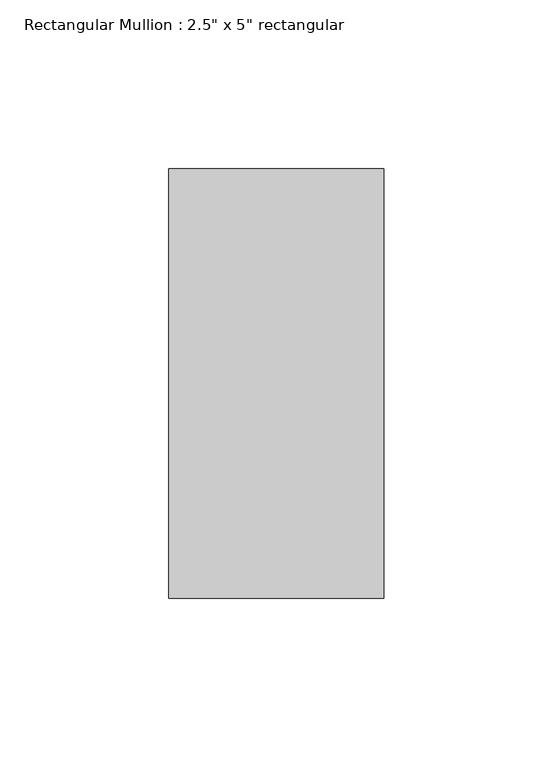
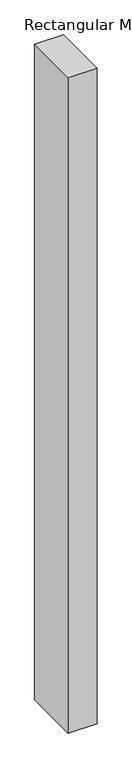
"""IFC4 building model written with IfcOpenShell, lengths in millimetres: member geometry."""

from ifc_helpers import new_model, si_unit, frame, origin, place, context, project, spatial, polyline, outline, extrude, source, transform, mapped, element, save


def member_fae4a232(model_context):
    return source(origin(), model_context, "Body", "SweptSolid", [
        extrude(outline(polyline([(31.75, 63.5), (31.75, -63.5), (-31.75, -63.5), (-31.75, 63.5), (31.75, 63.5)])), frame((0.0, 0.0, -1521.1896321), z_axis=(0.0, 0.0, 1.0), x_axis=(1.0, 0.0, 0.0)), (0.0, 0.0, 1.0), 1521.1896321),
    ])


if __name__ == "__main__":
    model = new_model("IFC4")
    model_context = context("Model", 3, world=origin())
    ifc_project = project(units=[si_unit("LENGTHUNIT", "METRE", prefix="MILLI")], contexts=[model_context])
    site = spatial("IfcSite", under=ifc_project)
    building = spatial("IfcBuilding", under=site)
    placement = place(None, origin())
    member_shape = member_fae4a232(model_context)
    element("IfcMember", 1, ObjectType="Rectangular Mullion : 2.5\" x 5\" rectangular", at=placement, inside=building, context=model_context, shape_type="MappedRepresentation", body=[
        mapped(member_shape, transform((0.0, 0.0, 0.0), x_axis=(1.0, 0.0, 0.0), y_axis=(0.0, 1.0, 0.0), z_axis=(0.0, 0.0, 1.0))),
    ])
    save(model, "model.ifc")

# Revit data of these elements
# Type "Rectangular Mullion : 2.5\" x 5\" rectangular"
#   built-in parameter 1007304 = 0.416667 (stored number, unit not read)
#   built-in parameter 1007301 = 0.104167 (stored number, unit not read)
#   built-in parameter 1007300 = 0.104167 (stored number, unit not read)
# Element 1 (IfcMember, "Rectangular Mullion : 2.5\" x 5\" rectangular")
#   Materials on its faces: "Aluminum"
# Materials
#   "Aluminum": class "Metal", colour RGB 247 247 247, transparency 0, Description = "Aluminum 6061", Cost = 0
